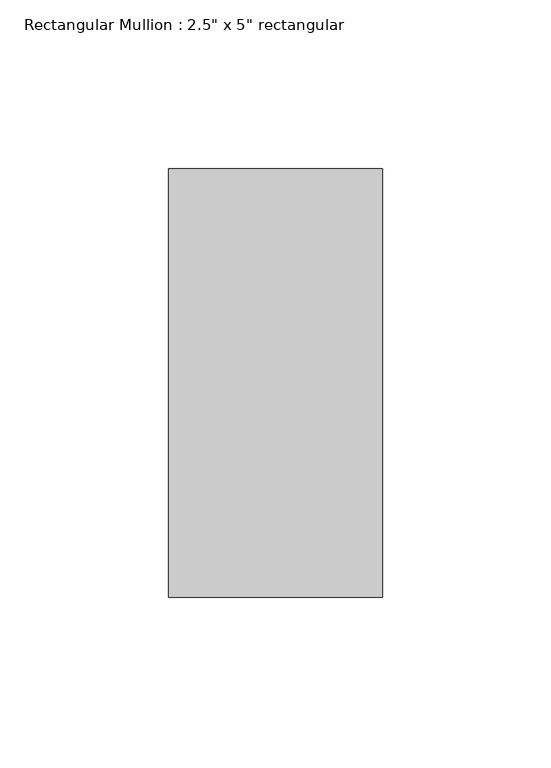
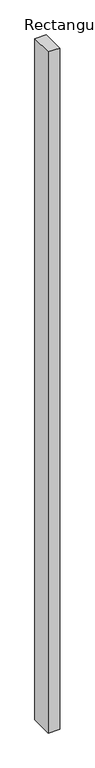
"""IFC4 building model written with IfcOpenShell, lengths in millimetres: member geometry."""

from ifc_helpers import new_model, si_unit, frame, origin, place, context, project, spatial, polyline, outline, extrude, source, transform, mapped, element, save


def member_5be86ab4(model_context):
    return source(origin(), model_context, "Body", "SweptSolid", [
        extrude(outline(polyline([(0.0, 63.5), (0.0, -63.5), (-63.5, -63.5), (-63.5, 63.5), (0.0, 63.5)])), frame((0.0, 0.0, -3962.4), z_axis=(0.0, 0.0, 1.0), x_axis=(1.0, 0.0, 0.0)), (0.0, 0.0, 1.0), 3962.4),
    ])


if __name__ == "__main__":
    model = new_model("IFC4")
    model_context = context("Model", 3, world=origin())
    ifc_project = project(units=[si_unit("LENGTHUNIT", "METRE", prefix="MILLI")], contexts=[model_context])
    site = spatial("IfcSite", under=ifc_project)
    building = spatial("IfcBuilding", under=site)
    placement = place(None, origin())
    member_shape = member_5be86ab4(model_context)
    element("IfcMember", 1, ObjectType="Rectangular Mullion : 2.5\" x 5\" rectangular", at=placement, inside=building, context=model_context, shape_type="MappedRepresentation", body=[
        mapped(member_shape, transform((0.0, 0.0, 0.0), x_axis=(1.0, 0.0, 0.0), y_axis=(0.0, 1.0, 0.0), z_axis=(0.0, 0.0, 1.0))),
    ])
    save(model, "model.ifc")

# Revit data of these elements
# Type "Rectangular Mullion : 2.5\" x 5\" rectangular"
#   built-in parameter 1007304 = 0.416667 (stored number, unit not read)
#   built-in parameter 1007301 = 0.104167 (stored number, unit not read)
#   built-in parameter 1007300 = 0.104167 (stored number, unit not read)
# Element 1 (IfcMember, "Rectangular Mullion : 2.5\" x 5\" rectangular")
#   Materials on its faces: "Iron, Ductile"
# Materials
#   "Iron, Ductile": class "Metal", colour RGB 0 0 0, transparency 0, Description = "Ductile cast iron", Cost = 0
